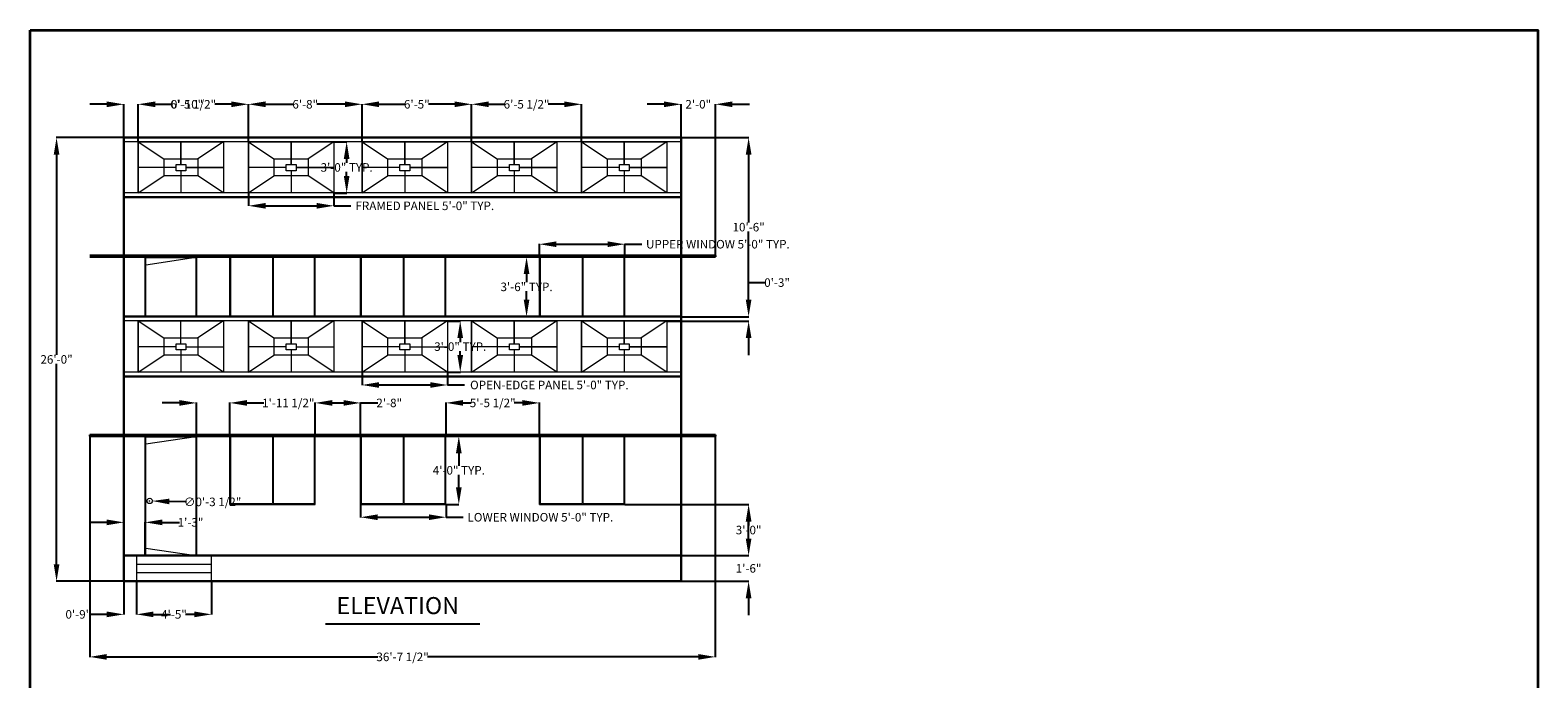
# Model space of a CAD drawing. Units: inches. Extents: x 115 to 1174, y 222 to 1302.
# Tile 5 of 5: x 115 to 1174, y 846 to 1302. Entities that reach past the tile are written whole.
import ezdxf

# ---------------------------------------------------------------- set-up
doc = ezdxf.new("R2010")
doc.units = ezdxf.units.IN
doc.header["$MEASUREMENT"] = 0
for name, color, linetype, lineweight in [('A-ANNO-DIMS', 2, 'Continuous', 18), ('A-ANNO-TEXT', 7, 'Continuous', 25), ('A-ANNO-TTLB', 7, 'Continuous', 35), ('A-ELEV', 7, 'Continuous', 30), ('A-ELEV-DOOR', 3, 'Continuous', 18), ('A-ELEV-GLAZ', 4, 'Continuous', 18), ('A-ELEV-PANL', 7, 'Continuous', 18), ('A-ELEV-STEP', 7, 'Continuous', 18)]:
    doc.layers.add(name, color=color, linetype=linetype, lineweight=lineweight)
doc.styles.get("Standard").update_dxf_attribs({"font": 'arial.ttf'})
doc.dimstyles.get("Standard").update_dxf_attribs({"dimtxt": 6, "dimasz": 12, "dimexe": 0.18, "dimexo": 0.0625, "dimgap": 0.09, "dimtad": 0, "dimtih": 1, "dimtoh": 1, "dimdec": 1, "dimzin": 0, "dimdsep": 46, "dimlunit": 3, "dimtxsty": 'Standard', "dimcen": 0.09, "dimadec": 0, "dimazin": 0, "dimtfac": 1, "dimtdec": 1, "dimtofl": 0, "dimtmove": 0, "dimatfit": 3, "dimfxl": 1, "dimtolj": 1, "dimtzin": 0, "dimarcsym": 0})

# ---------------------------------------------------------------- blocks, each defined once
blk = doc.blocks.new('FASCIA-PANEL-OPEN-EDGE')
for p, q in [((0, 36), (0, 0)), ((0, 36), (18, 24)), ((30, 20), (30, 36)), ((60, 36), (42, 24)), ((60, 36), (60, 0)), ((18, 24), (18, 12)), ((42, 24), (42, 12)), ((26.6, 17.8), (0, 17.8)), ((0, 0), (18, 12)), ((30, 15.6), (30, 0)), ((33.5, 17.8), (60, 17.8)), ((60, 0), (42, 12))]:
    blk.add_line(p, q)
for points in [[(60, 0), (0, 0), (0, 36), (60, 36)], [(18, 24), (42, 24)], [(42, 12), (18, 12)]]:
    blk.add_lwpolyline(points)
blk.add_lwpolyline([(26.6, 20), (33.5, 20), (33.5, 15.6), (26.6, 15.6)], close=True)
blk = doc.blocks.new('FASCIA-PANEL-FRAMED')
for p, q in [((0, 36), (0, 0)), ((0, 36), (18, 24)), ((30, 20), (30, 36)), ((60, 36), (42, 24)), ((60, 36), (60, 0)), ((18, 24), (18, 12)), ((42, 24), (42, 12)), ((26.6, 17.8), (0, 17.8)), ((0, 0), (18, 12)), ((30, 15.6), (30, 0)), ((33.5, 17.8), (60, 17.8)), ((60, 0), (42, 12))]:
    blk.add_line(p, q)
for points in [[(0, 36), (60, 36), (60, 0), (0, 0)], [(26.6, 20), (33.5, 20), (33.5, 15.6), (26.6, 15.6)]]:
    blk.add_lwpolyline(points, close=True)
for points in [[(18, 24), (42, 24)], [(42, 12), (18, 12)]]:
    blk.add_lwpolyline(points)
blk = doc.blocks.new('ELEV-WIN-TWIN-60X48')
for p, q in [((0, 48), (0, 0)), ((0, 0), (0, 48)), ((0.5, 47.5), (0.5, 0.5)), ((30, 47.5), (0.5, 47.5)), ((30, 47.5), (30, 0.5)), ((59.5, 47.5), (30.5, 47.5)), ((30.5, 47.5), (30.5, 0.5)), ((59.5, 0.5), (59.5, 47.5)), ((60, 0), (60, 48)), ((60, 0), (60, 48)), ((0.5, 0.5), (30, 0.5)), ((30.5, 0.5), (59.5, 0.5)), ((0, 0), (60, 0))]:
    blk.add_line(p, q)
blk = doc.blocks.new('ELEV-WIN-TWIN-60-UPPER')
for p, q in [((0, 42), (0, 0)), ((0, 0), (0, 42)), ((30, 41.5), (0.5, 41.5)), ((0.5, 41.5), (0.5, 0)), ((30, 41.5), (30, 0)), ((59.5, 41.5), (30.5, 41.5)), ((30.5, 41.5), (30.5, 0)), ((59.5, 0), (59.5, 41.5)), ((60, 0), (60, 42)), ((60, 0), (60, 42))]:
    blk.add_line(p, q)
blk = doc.blocks.new('*D29')
at = {"layer": 'A-ANNO-DIMS', "color": 0, "lineweight": -2, "transparency": 16777216}
for p, q in [((268.2, 1187.6), (268.2, 1178.5)), ((328.2, 1187.6), (328.2, 1178.5)), ((280.2, 1178.6), (316.2, 1178.6)), ((328.2, 1178.6), (340.2, 1178.6))]:
    blk.add_line(p, q, dxfattribs=at)
at = {"layer": 'A-ANNO-DIMS', "color": 0, "transparency": 16777216}
for points in [[(280.2, 1180.6), (280.2, 1176.6), (268.2, 1178.6)], [(316.2, 1180.6), (316.2, 1176.6), (328.2, 1178.6)]]:
    blk.add_solid(points, dxfattribs=at)
at = {"layer": 'Defpoints', "color": 0, "transparency": 16777216}
for p in [(268.2, 1187.6), (328.2, 1187.6), (328.2, 1178.6)]:
    blk.add_point(p, dxfattribs=at)
at = {"layer": 'A-ANNO-DIMS', "color": 0, "transparency": 16777216, "insert": (392.1, 1178.6), "char_height": 6, "attachment_point": 5}
blk.add_mtext('\\A1;FRAMED PANEL 5\'-0" TYP.', dxfattribs=at)
blk = doc.blocks.new('*D30')
at = {"layer": 'A-ANNO-DIMS', "color": 0, "lineweight": -2, "transparency": 16777216}
for p, q in [((328.2, 1223.6), (337.3, 1223.6)), ((337.2, 1211.6), (337.2, 1208.8)), ((337.2, 1199.6), (337.2, 1202.5)), ((328.2, 1187.6), (337.3, 1187.6))]:
    blk.add_line(p, q, dxfattribs=at)
at = {"layer": 'A-ANNO-DIMS', "color": 0, "transparency": 16777216}
for points in [[(335.2, 1211.6), (339.2, 1211.6), (337.2, 1223.6)], [(335.2, 1199.6), (339.2, 1199.6), (337.2, 1187.6)]]:
    blk.add_solid(points, dxfattribs=at)
at = {"layer": 'Defpoints', "color": 0, "transparency": 16777216}
for p in [(328.2, 1223.6), (337.2, 1223.6), (328.2, 1187.6)]:
    blk.add_point(p, dxfattribs=at)
at = {"layer": 'A-ANNO-DIMS', "color": 0, "transparency": 16777216, "insert": (337.2, 1205.6), "char_height": 6, "attachment_point": 5}
blk.add_mtext('\\A1;3\'-0" TYP.', dxfattribs=at)
blk = doc.blocks.new('*D31')
at = {"layer": 'A-ANNO-DIMS', "color": 0, "lineweight": -2, "transparency": 16777216}
for p, q in [((348, 1061.6), (348, 1052.5)), ((408, 1061.6), (408, 1052.5)), ((360, 1052.6), (396, 1052.6)), ((408, 1052.6), (420, 1052.6))]:
    blk.add_line(p, q, dxfattribs=at)
at = {"layer": 'A-ANNO-DIMS', "color": 0, "transparency": 16777216}
for points in [[(360, 1054.6), (360, 1050.6), (348, 1052.6)], [(396, 1054.6), (396, 1050.6), (408, 1052.6)]]:
    blk.add_solid(points, dxfattribs=at)
at = {"layer": 'Defpoints', "color": 0, "transparency": 16777216}
for p in [(348, 1061.6), (408, 1061.6), (408, 1052.6)]:
    blk.add_point(p, dxfattribs=at)
at = {"layer": 'A-ANNO-DIMS', "color": 0, "transparency": 16777216, "insert": (479.6, 1052.6), "char_height": 6, "attachment_point": 5}
blk.add_mtext('\\A1;OPEN-EDGE PANEL 5\'-0" TYP.', dxfattribs=at)
blk = doc.blocks.new('*D32')
at = {"layer": 'A-ANNO-DIMS', "color": 0, "lineweight": -2, "transparency": 16777216}
for p, q in [((408.1, 1097.6), (417.2, 1097.6)), ((417, 1085.6), (417, 1082.8)), ((417, 1073.6), (417, 1076.5)), ((408.1, 1061.6), (417.2, 1061.6))]:
    blk.add_line(p, q, dxfattribs=at)
at = {"layer": 'A-ANNO-DIMS', "color": 0, "transparency": 16777216}
for points in [[(415, 1085.6), (419, 1085.6), (417, 1097.6)], [(415, 1073.6), (419, 1073.6), (417, 1061.6)]]:
    blk.add_solid(points, dxfattribs=at)
at = {"layer": 'Defpoints', "color": 0, "transparency": 16777216}
for p in [(408, 1097.6), (417, 1097.6), (408, 1061.6)]:
    blk.add_point(p, dxfattribs=at)
at = {"layer": 'A-ANNO-DIMS', "color": 0, "transparency": 16777216, "insert": (417, 1079.6), "char_height": 6, "attachment_point": 5}
blk.add_mtext('\\A1;3\'-0" TYP.', dxfattribs=at)
blk = doc.blocks.new('*D33')
at = {"layer": 'A-ANNO-DIMS', "color": 0, "lineweight": -2, "transparency": 16777216}
for p, q in [((347, 968.6), (347, 959.5)), ((407, 968.6), (407, 959.5)), ((359, 959.6), (395, 959.6)), ((407, 959.6), (419, 959.6))]:
    blk.add_line(p, q, dxfattribs=at)
at = {"layer": 'A-ANNO-DIMS', "color": 0, "transparency": 16777216}
for points in [[(359, 961.6), (359, 957.6), (347, 959.6)], [(395, 961.6), (395, 957.6), (407, 959.6)]]:
    blk.add_solid(points, dxfattribs=at)
at = {"layer": 'Defpoints', "color": 0, "transparency": 16777216}
for p in [(347, 968.6), (407, 968.6), (407, 959.6)]:
    blk.add_point(p, dxfattribs=at)
at = {"layer": 'A-ANNO-DIMS', "color": 0, "transparency": 16777216, "insert": (473.3, 959.6), "char_height": 6, "attachment_point": 5}
blk.add_mtext('\\A1;LOWER WINDOW 5\'-0" TYP.', dxfattribs=at)
blk = doc.blocks.new('*D34')
at = {"layer": 'A-ANNO-DIMS', "color": 0, "lineweight": -2, "transparency": 16777216}
for p, q in [((407, 1016.6), (416.1, 1016.6)), ((416, 1004.6), (416, 995.8)), ((416, 980.6), (416, 989.5)), ((407, 968.6), (416.1, 968.6))]:
    blk.add_line(p, q, dxfattribs=at)
at = {"layer": 'A-ANNO-DIMS', "color": 0, "transparency": 16777216}
for points in [[(414, 1004.6), (418, 1004.6), (416, 1016.6)], [(414, 980.6), (418, 980.6), (416, 968.6)]]:
    blk.add_solid(points, dxfattribs=at)
at = {"layer": 'Defpoints', "color": 0, "transparency": 16777216}
for p in [(407, 1016.6), (416, 1016.6), (407, 968.6)]:
    blk.add_point(p, dxfattribs=at)
at = {"layer": 'A-ANNO-DIMS', "color": 0, "transparency": 16777216, "insert": (416, 992.6), "char_height": 6, "attachment_point": 5}
blk.add_mtext('\\A1;4\'-0" TYP.', dxfattribs=at)
blk = doc.blocks.new('*D35')
at = {"layer": 'A-ANNO-DIMS', "color": 0, "lineweight": -2, "transparency": 16777216}
for p, q in [((472.6, 1142.7), (472.6, 1151.8)), ((484.6, 1151.6), (520.6, 1151.6)), ((532.6, 1142.7), (532.6, 1151.8)), ((532.6, 1151.6), (544.6, 1151.6))]:
    blk.add_line(p, q, dxfattribs=at)
at = {"layer": 'A-ANNO-DIMS', "color": 0, "transparency": 16777216}
for points in [[(484.6, 1153.6), (484.6, 1149.6), (472.6, 1151.6)], [(520.6, 1153.6), (520.6, 1149.6), (532.6, 1151.6)]]:
    blk.add_solid(points, dxfattribs=at)
at = {"layer": 'Defpoints', "color": 0, "transparency": 16777216}
for p in [(532.6, 1151.6), (472.6, 1142.6), (532.6, 1142.6)]:
    blk.add_point(p, dxfattribs=at)
at = {"layer": 'A-ANNO-DIMS', "color": 0, "transparency": 16777216, "insert": (598, 1151.6), "char_height": 6, "attachment_point": 5}
blk.add_mtext('\\A1;UPPER WINDOW 5\'-0" TYP.', dxfattribs=at)
blk = doc.blocks.new('*D36')
at = {"layer": 'A-ANNO-DIMS', "color": 0, "lineweight": -2, "transparency": 16777216}
for p, q in [((472.5, 1142.6), (463.4, 1142.6)), ((463.6, 1130.6), (463.6, 1124.8)), ((463.6, 1112.6), (463.6, 1118.5)), ((472.5, 1100.6), (463.4, 1100.6))]:
    blk.add_line(p, q, dxfattribs=at)
at = {"layer": 'A-ANNO-DIMS', "color": 0, "transparency": 16777216}
for points in [[(461.6, 1130.6), (465.6, 1130.6), (463.6, 1142.6)], [(461.6, 1112.6), (465.6, 1112.6), (463.6, 1100.6)]]:
    blk.add_solid(points, dxfattribs=at)
at = {"layer": 'Defpoints', "color": 0, "transparency": 16777216}
for p in [(463.6, 1142.6), (472.6, 1142.6), (472.6, 1100.6)]:
    blk.add_point(p, dxfattribs=at)
at = {"layer": 'A-ANNO-DIMS', "color": 0, "transparency": 16777216, "insert": (463.6, 1121.6), "char_height": 6, "attachment_point": 5}
blk.add_mtext('\\A1;3\'-6" TYP.', dxfattribs=at)
blk = doc.blocks.new('*D71')
at = {"layer": 'A-ANNO-DIMS', "color": 0, "lineweight": -2, "transparency": 16777216}
for p, q in [((156.7, 1017.6), (156.7, 861.2)), ((596.2, 1017.6), (596.2, 861.2)), ((168.7, 861.4), (359.1, 861.4)), ((584.2, 861.4), (393.9, 861.4))]:
    blk.add_line(p, q, dxfattribs=at)
at = {"layer": 'A-ANNO-DIMS', "color": 0, "transparency": 16777216}
for points in [[(168.7, 863.4), (168.7, 859.4), (156.7, 861.4)], [(584.2, 863.4), (584.2, 859.4), (596.2, 861.4)]]:
    blk.add_solid(points, dxfattribs=at)
at = {"layer": 'Defpoints', "color": 0, "transparency": 16777216}
for p in [(156.7, 1017.6), (596.2, 1017.6), (596.2, 861.4)]:
    blk.add_point(p, dxfattribs=at)
at = {"layer": 'A-ANNO-DIMS', "color": 0, "transparency": 16777216, "insert": (376.5, 861.4), "char_height": 6, "attachment_point": 5}
blk.add_mtext('\\A1;36\'-7 1/2"', dxfattribs=at)
blk = doc.blocks.new('*D72')
at = {"layer": 'A-ANNO-DIMS', "color": 0, "lineweight": -2, "transparency": 16777216}
for p, q in [((180.7, 1226.6), (133.2, 1226.6)), ((133.4, 1214.6), (133.4, 1073.8)), ((133.4, 926.6), (133.4, 1067.5)), ((180.7, 914.6), (133.2, 914.6))]:
    blk.add_line(p, q, dxfattribs=at)
at = {"layer": 'A-ANNO-DIMS', "color": 0, "transparency": 16777216}
for points in [[(131.4, 1214.6), (135.4, 1214.6), (133.4, 1226.6)], [(131.4, 926.6), (135.4, 926.6), (133.4, 914.6)]]:
    blk.add_solid(points, dxfattribs=at)
at = {"layer": 'Defpoints', "color": 0, "transparency": 16777216}
for p in [(133.4, 1226.6), (180.7, 1226.6), (180.7, 914.6)]:
    blk.add_point(p, dxfattribs=at)
at = {"layer": 'A-ANNO-DIMS', "color": 0, "transparency": 16777216, "insert": (133.4, 1070.6), "char_height": 6, "attachment_point": 5}
blk.add_mtext('\\A1;26\'-0"', dxfattribs=at)
blk = doc.blocks.new('*D73')
at = {"layer": 'A-ANNO-DIMS', "color": 0, "lineweight": -2, "transparency": 16777216}
for p, q in [((560.219665, 1249.999861), (548.219665, 1249.999861)), ((572.219665, 1226.712361), (572.219665, 1250.179861)), ((596.219665, 1143.712361), (596.219665, 1250.179861)), ((608.219665, 1249.999861), (620.219665, 1249.999861))]:
    blk.add_line(p, q, dxfattribs=at)
at = {"layer": 'A-ANNO-DIMS', "color": 0, "transparency": 16777216}
for points in [[(560.219665, 1251.999861), (560.219665, 1247.999861), (572.219665, 1249.999861)], [(608.219665, 1251.999861), (608.219665, 1247.999861), (596.219665, 1249.999861)]]:
    blk.add_solid(points, dxfattribs=at)
at = {"layer": 'Defpoints', "color": 0, "transparency": 16777216}
for p in [(572.219665, 1249.999861), (572.219665, 1226.649861), (596.219665, 1143.649861)]:
    blk.add_point(p, dxfattribs=at)
at = {"layer": 'A-ANNO-DIMS', "color": 0, "transparency": 16777216, "insert": (584.219665, 1249.999861), "char_height": 6, "attachment_point": 5}
blk.add_mtext('\\A1;2\'-0"', dxfattribs=at)
blk = doc.blocks.new('*D74')
at = {"layer": 'A-ANNO-DIMS', "color": 0, "lineweight": -2, "transparency": 16777216}
for p, q in [((168.7, 1250), (156.7, 1250)), ((180.7, 1226.7), (180.7, 1250.2)), ((190.7, 1223.7), (190.7, 1250.2)), ((202.7, 1250), (214.7, 1250))]:
    blk.add_line(p, q, dxfattribs=at)
at = {"layer": 'A-ANNO-DIMS', "color": 0, "transparency": 16777216}
for points in [[(168.7, 1252), (168.7, 1248), (180.7, 1250)], [(202.7, 1252), (202.7, 1248), (190.7, 1250)]]:
    blk.add_solid(points, dxfattribs=at)
at = {"layer": 'Defpoints', "color": 0, "transparency": 16777216}
for p in [(190.7, 1250), (180.7, 1226.6), (190.7, 1223.6)]:
    blk.add_point(p, dxfattribs=at)
at = {"layer": 'A-ANNO-DIMS', "color": 0, "transparency": 16777216, "insert": (225.1, 1250), "char_height": 6, "attachment_point": 5}
blk.add_mtext('\\A1;0\'-10"', dxfattribs=at)
blk = doc.blocks.new('*D75')
at = {"layer": 'A-ANNO-DIMS', "color": 0, "lineweight": -2, "transparency": 16777216}
for p, q in [((190.7, 1223.7), (190.7, 1250.2)), ((202.7, 1250), (214.4, 1250)), ((256.2, 1250), (244.5, 1250)), ((268.2, 1223.7), (268.2, 1250.2))]:
    blk.add_line(p, q, dxfattribs=at)
at = {"layer": 'A-ANNO-DIMS', "color": 0, "transparency": 16777216}
for points in [[(202.7, 1252), (202.7, 1248), (190.7, 1250)], [(256.2, 1252), (256.2, 1248), (268.2, 1250)]]:
    blk.add_solid(points, dxfattribs=at)
at = {"layer": 'Defpoints', "color": 0, "transparency": 16777216}
for p in [(268.2, 1250), (190.7, 1223.6), (268.2, 1223.6)]:
    blk.add_point(p, dxfattribs=at)
at = {"layer": 'A-ANNO-DIMS', "color": 0, "transparency": 16777216, "insert": (229.4, 1250), "char_height": 6, "attachment_point": 5}
blk.add_mtext('\\A1;6\'-5 1/2"', dxfattribs=at)
blk = doc.blocks.new('*D76')
at = {"layer": 'A-ANNO-DIMS', "color": 0, "lineweight": -2, "transparency": 16777216}
for p, q in [((268.2, 1223.7), (268.2, 1250.2)), ((280.2, 1250), (300, 1250)), ((336, 1250), (316.2, 1250)), ((348, 1223.7), (348, 1250.2))]:
    blk.add_line(p, q, dxfattribs=at)
at = {"layer": 'A-ANNO-DIMS', "color": 0, "transparency": 16777216}
for points in [[(280.2, 1252), (280.2, 1248), (268.2, 1250)], [(336, 1252), (336, 1248), (348, 1250)]]:
    blk.add_solid(points, dxfattribs=at)
at = {"layer": 'Defpoints', "color": 0, "transparency": 16777216}
for p in [(348, 1250), (268.2, 1223.6), (348, 1223.6)]:
    blk.add_point(p, dxfattribs=at)
at = {"layer": 'A-ANNO-DIMS', "color": 0, "transparency": 16777216, "insert": (308.1, 1250), "char_height": 6, "attachment_point": 5}
blk.add_mtext('\\A1;6\'-8"', dxfattribs=at)
blk = doc.blocks.new('*D77')
at = {"layer": 'A-ANNO-DIMS', "color": 0, "lineweight": -2, "transparency": 16777216}
for p, q in [((348, 1223.7), (348, 1250.2)), ((360, 1250), (378.4, 1250)), ((413, 1250), (394.6, 1250)), ((425, 1223.7), (425, 1250.2))]:
    blk.add_line(p, q, dxfattribs=at)
at = {"layer": 'A-ANNO-DIMS', "color": 0, "transparency": 16777216}
for points in [[(360, 1252), (360, 1248), (348, 1250)], [(413, 1252), (413, 1248), (425, 1250)]]:
    blk.add_solid(points, dxfattribs=at)
at = {"layer": 'Defpoints', "color": 0, "transparency": 16777216}
for p in [(425, 1250), (348, 1223.6), (425, 1223.6)]:
    blk.add_point(p, dxfattribs=at)
at = {"layer": 'A-ANNO-DIMS', "color": 0, "transparency": 16777216, "insert": (386.5, 1250), "char_height": 6, "attachment_point": 5}
blk.add_mtext('\\A1;6\'-5"', dxfattribs=at)
blk = doc.blocks.new('*D78')
at = {"layer": 'A-ANNO-DIMS', "color": 0, "lineweight": -2, "transparency": 16777216}
for p, q in [((425, 1223.7), (425, 1250.2)), ((437, 1250), (448.5, 1250)), ((490.2, 1250), (478.7, 1250)), ((502.2, 1223.7), (502.2, 1250.2))]:
    blk.add_line(p, q, dxfattribs=at)
at = {"layer": 'A-ANNO-DIMS', "color": 0, "transparency": 16777216}
for points in [[(437, 1252), (437, 1248), (425, 1250)], [(490.2, 1252), (490.2, 1248), (502.2, 1250)]]:
    blk.add_solid(points, dxfattribs=at)
at = {"layer": 'Defpoints', "color": 0, "transparency": 16777216}
for p in [(502.2, 1250), (425, 1223.6), (502.2, 1223.6)]:
    blk.add_point(p, dxfattribs=at)
at = {"layer": 'A-ANNO-DIMS', "color": 0, "transparency": 16777216, "insert": (463.6, 1250), "char_height": 6, "attachment_point": 5}
blk.add_mtext('\\A1;6\'-5 1/2"', dxfattribs=at)
blk = doc.blocks.new('*D79')
at = {"layer": 'A-ANNO-DIMS', "color": 0, "lineweight": -2, "transparency": 16777216}
for p, q in [((180.7, 914.6), (180.7, 891.1)), ((189.5, 914.6), (189.5, 891.1)), ((168.7, 891.3), (156.7, 891.3)), ((201.5, 891.3), (213.5, 891.3))]:
    blk.add_line(p, q, dxfattribs=at)
at = {"layer": 'A-ANNO-DIMS', "color": 0, "transparency": 16777216}
for points in [[(168.7, 893.3), (168.7, 889.3), (180.7, 891.3)], [(201.5, 893.3), (201.5, 889.3), (189.5, 891.3)]]:
    blk.add_solid(points, dxfattribs=at)
at = {"layer": 'Defpoints', "color": 0, "transparency": 16777216}
for p in [(180.7, 914.6), (189.5, 914.6), (180.7, 891.3)]:
    blk.add_point(p, dxfattribs=at)
at = {"layer": 'A-ANNO-DIMS', "color": 0, "transparency": 16777216, "insert": (148.7, 891.3), "char_height": 6, "attachment_point": 5}
blk.add_mtext('\\A1;0\'-9"', dxfattribs=at)
blk = doc.blocks.new('*D80')
at = {"layer": 'A-ANNO-DIMS', "color": 0, "lineweight": -2, "transparency": 16777216}
for p, q in [((189.5, 914.6), (189.5, 891.1)), ((242.3, 914.6), (242.3, 891.1)), ((201.5, 891.3), (207.7, 891.3)), ((230.3, 891.3), (224.1, 891.3))]:
    blk.add_line(p, q, dxfattribs=at)
at = {"layer": 'A-ANNO-DIMS', "color": 0, "transparency": 16777216}
for points in [[(201.5, 893.3), (201.5, 889.3), (189.5, 891.3)], [(230.3, 893.3), (230.3, 889.3), (242.3, 891.3)]]:
    blk.add_solid(points, dxfattribs=at)
at = {"layer": 'Defpoints', "color": 0, "transparency": 16777216}
for p in [(189.5, 914.6), (242.3, 914.6), (189.5, 891.3)]:
    blk.add_point(p, dxfattribs=at)
at = {"layer": 'A-ANNO-DIMS', "color": 0, "transparency": 16777216, "insert": (215.9, 891.3), "char_height": 6, "attachment_point": 5}
blk.add_mtext('\\A1;4\'-5"', dxfattribs=at)
blk = doc.blocks.new('*D81')
at = {"layer": 'A-ANNO-DIMS', "color": 0, "lineweight": -2, "transparency": 16777216}
for p, q in [((168.7, 956), (156.7, 956)), ((180.7, 932.7), (180.7, 956.2)), ((195.7, 932.7), (195.7, 956.2)), ((207.7, 956), (219.7, 956))]:
    blk.add_line(p, q, dxfattribs=at)
at = {"layer": 'A-ANNO-DIMS', "color": 0, "transparency": 16777216}
for points in [[(168.7, 958), (168.7, 954), (180.7, 956)], [(207.7, 958), (207.7, 954), (195.7, 956)]]:
    blk.add_solid(points, dxfattribs=at)
at = {"layer": 'Defpoints', "color": 0, "transparency": 16777216}
for p in [(195.7, 956), (180.7, 932.6), (195.7, 932.6)]:
    blk.add_point(p, dxfattribs=at)
at = {"layer": 'A-ANNO-DIMS', "color": 0, "transparency": 16777216, "insert": (227.5, 956), "char_height": 6, "attachment_point": 5}
blk.add_mtext('\\A1;1\'-3"', dxfattribs=at)
blk = doc.blocks.new('*D82')
at = {"layer": 'A-ANNO-DIMS', "color": 0, "lineweight": -2, "transparency": 16777216}
for p, q in [((219.7, 1040), (207.7, 1040)), ((231.7, 1016.7), (231.7, 1040.2)), ((255.1, 1016.7), (255.1, 1040.2)), ((267.1, 1040), (279.1, 1040))]:
    blk.add_line(p, q, dxfattribs=at)
at = {"layer": 'A-ANNO-DIMS', "color": 0, "transparency": 16777216}
for points in [[(219.7, 1042), (219.7, 1038), (231.7, 1040)], [(267.1, 1042), (267.1, 1038), (255.1, 1040)]]:
    blk.add_solid(points, dxfattribs=at)
at = {"layer": 'Defpoints', "color": 0, "transparency": 16777216}
for p in [(255.1, 1040), (231.7, 1016.6), (255.1, 1016.6)]:
    blk.add_point(p, dxfattribs=at)
at = {"layer": 'A-ANNO-DIMS', "color": 0, "transparency": 16777216, "insert": (296.2, 1040), "char_height": 6, "attachment_point": 5}
blk.add_mtext('\\A1;1\'-11 1/2"', dxfattribs=at)
blk = doc.blocks.new('*D83')
at = {"layer": 'A-ANNO-DIMS', "color": 0, "lineweight": -2, "transparency": 16777216}
for p, q in [((315.1, 1016.7), (315.1, 1040.2)), ((327.1, 1040), (335, 1040)), ((347, 1016.7), (347, 1040.2)), ((347, 1040), (359, 1040))]:
    blk.add_line(p, q, dxfattribs=at)
at = {"layer": 'A-ANNO-DIMS', "color": 0, "transparency": 16777216}
for points in [[(327.1, 1042), (327.1, 1038), (315.1, 1040)], [(335, 1042), (335, 1038), (347, 1040)]]:
    blk.add_solid(points, dxfattribs=at)
at = {"layer": 'Defpoints', "color": 0, "transparency": 16777216}
for p in [(347, 1040), (315.1, 1016.6), (347, 1016.6)]:
    blk.add_point(p, dxfattribs=at)
at = {"layer": 'A-ANNO-DIMS', "color": 0, "transparency": 16777216, "insert": (367.1, 1040), "char_height": 6, "attachment_point": 5}
blk.add_mtext('\\A1;2\'-8"', dxfattribs=at)
blk = doc.blocks.new('*D84')
at = {"layer": 'A-ANNO-DIMS', "color": 0, "lineweight": -2, "transparency": 16777216}
for p, q in [((407, 1016.7), (407, 1040.2)), ((419, 1040), (424.7, 1040)), ((460.6, 1040), (454.8, 1040)), ((472.6, 1016.7), (472.6, 1040.2))]:
    blk.add_line(p, q, dxfattribs=at)
at = {"layer": 'A-ANNO-DIMS', "color": 0, "transparency": 16777216}
for points in [[(419, 1042), (419, 1038), (407, 1040)], [(460.6, 1042), (460.6, 1038), (472.6, 1040)]]:
    blk.add_solid(points, dxfattribs=at)
at = {"layer": 'Defpoints', "color": 0, "transparency": 16777216}
for p in [(472.6, 1040), (407, 1016.6), (472.6, 1016.6)]:
    blk.add_point(p, dxfattribs=at)
at = {"layer": 'A-ANNO-DIMS', "color": 0, "transparency": 16777216, "insert": (439.8, 1040), "char_height": 6, "attachment_point": 5}
blk.add_mtext('\\A1;5\'-5 1/2"', dxfattribs=at)
blk = doc.blocks.new('*D85')
at = {"layer": 'A-ANNO-DIMS', "color": 0, "lineweight": -2, "transparency": 16777216}
for p, q in [((619.569665, 944.649861), (619.569665, 956.649861)), ((572.282165, 932.649861), (619.749665, 932.649861)), ((572.282165, 914.649861), (619.749665, 914.649861)), ((619.569665, 902.649861), (619.569665, 890.649861))]:
    blk.add_line(p, q, dxfattribs=at)
at = {"layer": 'A-ANNO-DIMS', "color": 0, "transparency": 16777216}
for points in [[(617.569665, 944.649861), (621.569665, 944.649861), (619.569665, 932.649861)], [(617.569665, 902.649861), (621.569665, 902.649861), (619.569665, 914.649861)]]:
    blk.add_solid(points, dxfattribs=at)
at = {"layer": 'Defpoints', "color": 0, "transparency": 16777216}
for p in [(572.219665, 932.649861), (619.569665, 932.649861), (572.219665, 914.649861)]:
    blk.add_point(p, dxfattribs=at)
at = {"layer": 'A-ANNO-DIMS', "color": 0, "transparency": 16777216, "insert": (619.569665, 923.649861), "char_height": 6, "attachment_point": 5}
blk.add_mtext('\\A1;1\'-6"', dxfattribs=at)
blk = doc.blocks.new('*D86')
at = {"layer": 'A-ANNO-DIMS', "color": 0, "lineweight": -2, "transparency": 16777216}
for p, q in [((532.7, 968.6), (619.7, 968.6)), ((619.6, 956.6), (619.6, 953.8)), ((619.6, 944.6), (619.6, 947.5)), ((572.3, 932.6), (619.7, 932.6))]:
    blk.add_line(p, q, dxfattribs=at)
at = {"layer": 'A-ANNO-DIMS', "color": 0, "transparency": 16777216}
for points in [[(617.6, 956.6), (621.6, 956.6), (619.6, 968.6)], [(617.6, 944.6), (621.6, 944.6), (619.6, 932.6)]]:
    blk.add_solid(points, dxfattribs=at)
at = {"layer": 'Defpoints', "color": 0, "transparency": 16777216}
for p in [(532.6, 968.6), (619.6, 968.6), (572.2, 932.6)]:
    blk.add_point(p, dxfattribs=at)
at = {"layer": 'A-ANNO-DIMS', "color": 0, "transparency": 16777216, "insert": (619.6, 950.6), "char_height": 6, "attachment_point": 5}
blk.add_mtext('\\A1;3\'-0"', dxfattribs=at)
blk = doc.blocks.new('*D87')
at = {"layer": 'A-ANNO-DIMS', "color": 0, "lineweight": -2, "transparency": 16777216}
for p, q in [((572.3, 1226.6), (619.7, 1226.6)), ((619.6, 1214.6), (619.6, 1166.8)), ((619.6, 1112.6), (619.6, 1160.5)), ((572.3, 1100.6), (619.7, 1100.6))]:
    blk.add_line(p, q, dxfattribs=at)
at = {"layer": 'A-ANNO-DIMS', "color": 0, "transparency": 16777216}
for points in [[(617.6, 1214.6), (621.6, 1214.6), (619.6, 1226.6)], [(617.6, 1112.6), (621.6, 1112.6), (619.6, 1100.6)]]:
    blk.add_solid(points, dxfattribs=at)
at = {"layer": 'Defpoints', "color": 0, "transparency": 16777216}
for p in [(572.2, 1226.6), (619.6, 1226.6), (572.2, 1100.6)]:
    blk.add_point(p, dxfattribs=at)
at = {"layer": 'A-ANNO-DIMS', "color": 0, "transparency": 16777216, "insert": (619.6, 1163.6), "char_height": 6, "attachment_point": 5}
blk.add_mtext('\\A1;10\'-6"', dxfattribs=at)
blk = doc.blocks.new('*D88')
at = {"layer": 'A-ANNO-DIMS', "color": 0, "lineweight": -2, "transparency": 16777216}
for p, q in [((619.6, 1112.6), (619.6, 1124.6)), ((619.6, 1124.6), (631.6, 1124.6)), ((562.3, 1097.6), (619.7, 1097.6)), ((572.3, 1100.6), (619.7, 1100.6)), ((619.6, 1085.6), (619.6, 1073.6))]:
    blk.add_line(p, q, dxfattribs=at)
at = {"layer": 'A-ANNO-DIMS', "color": 0, "transparency": 16777216}
for points in [[(617.6, 1112.6), (621.6, 1112.6), (619.6, 1100.6)], [(617.6, 1085.6), (621.6, 1085.6), (619.6, 1097.6)]]:
    blk.add_solid(points, dxfattribs=at)
at = {"layer": 'Defpoints', "color": 0, "transparency": 16777216}
for p in [(562.2, 1097.6), (572.2, 1100.6), (619.6, 1100.6)]:
    blk.add_point(p, dxfattribs=at)
at = {"layer": 'A-ANNO-DIMS', "color": 0, "transparency": 16777216, "insert": (639.6, 1124.6), "char_height": 6, "attachment_point": 5}
blk.add_mtext('\\A1;0\'-3"', dxfattribs=at)
blk = doc.blocks.new('*D98')
at = {"layer": 'A-ANNO-DIMS', "color": 0, "lineweight": -2, "transparency": 16777216}
for p, q in [((198.7, 971.1), (198.9, 971.1)), ((198.8, 971), (198.8, 971.1)), ((224.7, 970.4), (212.7, 970.7))]:
    blk.add_line(p, q, dxfattribs=at)
at = {"layer": 'A-ANNO-DIMS', "color": 0, "transparency": 16777216}
blk.add_solid([(212.7, 972.7), (212.6, 968.7), (200.7, 971)], dxfattribs=at)
at = {"layer": 'Defpoints', "color": 0, "transparency": 16777216}
for p in [(197, 971.1), (200.7, 971)]:
    blk.add_point(p, dxfattribs=at)
at = {"layer": 'A-ANNO-DIMS', "color": 0, "transparency": 16777216, "insert": (243, 970.4), "char_height": 6, "attachment_point": 5}
blk.add_mtext('\\A1;∅0\'-3 1/2"', dxfattribs=at)

msp = doc.modelspace()

# ---------------------------------------------------------------- linework, layer by layer
at = {"layer": 'A-ANNO-TEXT'}
msp.add_line((322.46, 884.76), (430.72, 884.76), dxfattribs=at)
at = {"layer": 'A-ANNO-TTLB'}
msp.add_lwpolyline([(114.85, 1302.15), (1174.06, 1302.15), (1174.06, 222.13), (114.85, 222.13)], close=True, dxfattribs=at)
at = {"layer": 'A-ELEV'}
for p, q in [((572.22, 1226.65), (180.72, 1226.65)), ((180.72, 1097.65), (180.72, 1226.65)), ((572.22, 1040.65), (572.22, 1226.65)), ((572.22, 1184.65), (180.72, 1184.65)), ((156.72, 1143.65), (572.22, 1143.65)), ((180.72, 1142.65), (156.72, 1142.65)), ((572.22, 1142.65), (180.72, 1142.65)), ((572.22, 1143.65), (596.22, 1143.65)), ((596.22, 1142.65), (572.22, 1142.65)), ((596.22, 1143.65), (596.22, 1142.65)), ((180.72, 914.65), (180.72, 1100.65)), ((572.22, 1100.65), (180.72, 1100.65)), ((572.22, 914.65), (572.22, 1100.65)), ((572.22, 1058.65), (180.72, 1058.65)), ((156.72, 1016.65), (156.72, 1017.65)), ((156.72, 1017.65), (572.22, 1017.65)), ((572.22, 1017.65), (596.22, 1017.65)), ((596.22, 1017.65), (596.22, 1016.65)), ((180.72, 1016.65), (156.72, 1016.65)), ((572.22, 1016.65), (180.72, 1016.65)), ((596.22, 1016.65), (572.22, 1016.65)), ((572.22, 932.65), (180.72, 932.65)), ((572.22, 914.65), (180.72, 914.65))]:
    msp.add_line(p, q, dxfattribs=at)
at = {"layer": 'A-ELEV-DOOR'}
for p, q in [((195.72, 1142.65), (231.72, 1142.65)), ((195.72, 1100.65), (195.72, 1142.65)), ((195.72, 1100.65), (195.72, 1142.65)), ((196.22, 1142.15), (231.22, 1142.15)), ((196.22, 1100.65), (196.22, 1142.15)), ((231.22, 1142.15), (196.22, 1136.89)), ((231.22, 1142.15), (231.22, 1100.65)), ((231.72, 1142.65), (231.72, 1100.65)), ((231.72, 1100.65), (231.72, 1142.65)), ((195.72, 932.65), (195.72, 1016.65)), ((195.72, 932.65), (195.72, 1016.65)), ((195.72, 1016.65), (231.72, 1016.65)), ((196.22, 932.65), (196.22, 1016.15)), ((196.22, 1016.15), (231.22, 1016.15)), ((231.22, 1016.15), (196.22, 1010.89)), ((231.22, 1016.15), (231.22, 932.65)), ((231.72, 932.65), (231.72, 1016.65)), ((231.72, 1016.65), (231.72, 932.65)), ((196.22, 932.65), (196.22, 937.95)), ((196.22, 937.95), (231.22, 932.65))]:
    msp.add_line(p, q, dxfattribs=at)
msp.add_circle((198.83, 971.05), 1.87, dxfattribs=at)
at = {"layer": 'A-ELEV-GLAZ'}
for p, q in [((406.96, 1142.65), (346.96, 1142.65)), ((532.61, 1142.65), (472.61, 1142.65)), ((406.96, 1016.65), (346.96, 1016.65)), ((532.61, 1016.65), (472.61, 1016.65))]:
    msp.add_line(p, q, dxfattribs=at)
at = {"layer": 'A-ELEV-PANL'}
for p, q in [((572.22, 1223.65), (180.72, 1223.65)), ((180.72, 1223.65), (180.72, 1187.65)), ((220.72, 1223.65), (220.72, 1207.7)), ((298.15, 1223.65), (298.15, 1207.7)), ((378.01, 1223.65), (378.01, 1207.7)), ((454.96, 1223.65), (454.96, 1207.7)), ((532.22, 1223.65), (532.22, 1207.7)), ((562.22, 1223.65), (562.22, 1187.65)), ((572.22, 1223.65), (572.22, 1187.65)), ((250.72, 1205.45), (224.25, 1205.45)), ((328.15, 1205.45), (301.69, 1205.45)), ((408.01, 1205.45), (381.55, 1205.45)), ((484.96, 1205.45), (458.49, 1205.45)), ((562.22, 1205.45), (535.75, 1205.45)), ((572.22, 1187.65), (180.72, 1187.65)), ((572.22, 1097.65), (180.72, 1097.65)), ((180.72, 1097.65), (180.72, 1061.65)), ((298.15, 1097.65), (298.15, 1081.7)), ((378.01, 1097.65), (378.01, 1081.7)), ((454.96, 1097.65), (454.96, 1081.7)), ((532.22, 1097.65), (532.22, 1081.7)), ((562.22, 1097.65), (562.22, 1061.65)), ((572.22, 1097.65), (572.22, 1061.65)), ((484.96, 1079.45), (458.49, 1079.45)), ((562.22, 1079.45), (535.75, 1079.45)), ((572.22, 1061.65), (180.72, 1061.65)), ((180.72, 1058.65), (180.72, 1061.65))]:
    msp.add_line(p, q, dxfattribs=at)
at = {"layer": 'A-ELEV-STEP'}
for p, q in [((189.5, 932.65), (189.5, 914.65)), ((242.31, 932.65), (189.5, 932.65)), ((242.31, 914.65), (242.31, 932.65)), ((189.5, 926.65), (242.31, 926.65)), ((189.5, 920.65), (242.31, 920.65)), ((189.5, 914.65), (242.31, 914.65))]:
    msp.add_line(p, q, dxfattribs=at)

# ---------------------------------------------------------------- block references
at = {"layer": 'A-ELEV-GLAZ'}
for name, p in [('ELEV-WIN-TWIN-60-UPPER', (255.09, 1100.65)), ('ELEV-WIN-TWIN-60-UPPER', (346.96, 1100.65)), ('ELEV-WIN-TWIN-60-UPPER', (472.61, 1100.65)), ('ELEV-WIN-TWIN-60X48', (255.09, 968.65)), ('ELEV-WIN-TWIN-60X48', (346.96, 968.65)), ('ELEV-WIN-TWIN-60X48', (472.61, 968.65))]:
    msp.add_blockref(name, p, dxfattribs=at)
at = {"layer": 'A-ELEV-PANL'}
for name, p in [('FASCIA-PANEL-FRAMED', (190.72, 1187.65)), ('FASCIA-PANEL-FRAMED', (268.16, 1187.65)), ('FASCIA-PANEL-FRAMED', (348.01, 1187.65)), ('FASCIA-PANEL-FRAMED', (424.96, 1187.65)), ('FASCIA-PANEL-FRAMED', (502.22, 1187.65)), ('FASCIA-PANEL-OPEN-EDGE', (190.72, 1061.65)), ('FASCIA-PANEL-OPEN-EDGE', (268.16, 1061.65)), ('FASCIA-PANEL-OPEN-EDGE', (348.01, 1061.65)), ('FASCIA-PANEL-FRAMED', (424.96, 1061.65)), ('FASCIA-PANEL-FRAMED', (502.22, 1061.65))]:
    msp.add_blockref(name, p, dxfattribs=at)

# ---------------------------------------------------------------- texts
at = {"layer": 'A-ANNO-TEXT', "insert": (330.02, 903.46), "char_height": 12, "attachment_point": 1}
msp.add_mtext_dynamic_manual_height_columns('ELEVATION', width=186.2726, gutter_width=30, heights=[0], dxfattribs=at)

# ---------------------------------------------------------------- dimensions: what is measured, and where the dimension line sits
at = {"layer": 'A-ANNO-DIMS'}
for base, p1, p2, picture, middle in [((190.72, 1250), (180.72, 1226.65), (190.72, 1223.65), '*D74', (225.12, 1250)), ((268.15, 1250), (190.72, 1223.65), (268.15, 1223.65), '*D75', (229.44, 1250)), ((348.01, 1250), (268.15, 1223.65), (348.01, 1223.65), '*D76', (308.08, 1250)), ((424.9597, 1249.9999), (348.0128, 1223.6499), (424.9597, 1223.6499), '*D77', (386.4862, 1249.9999)), ((502.22, 1250), (424.96, 1223.65), (502.22, 1223.65), '*D78', (463.59, 1250)), ((572.22, 1250), (596.22, 1143.65), (572.22, 1226.65), '*D73', (584.22, 1250)), ((346.96, 1040), (315.09, 1016.65), (346.96, 1016.65), '*D83', (367.07, 1040)), ((596.22, 861.41), (156.72, 1017.65), (596.22, 1017.65), '*D71', (376.47, 861.41))]:
    dim = msp.add_linear_dim(base=base, p1=p1, p2=p2, dimstyle='Standard', override={"dimdec": 1, "dimlfac": 1, "dimrnd": 0, "dimzin": 1, "dimdsep": 46, "dimlunit": 4, "dimfrac": 2}, dxfattribs=at)
    dim.commit()
    dim.dimension.update_dxf_attribs({"geometry": picture, "text_midpoint": middle})
for base, p1, p2, angle, picture, middle in [((133.37, 1226.65), (180.72, 914.65), (180.72, 1226.65), 90, '*D72', (133.37, 1070.65)), ((619.57, 1226.65), (572.22, 1100.65), (572.22, 1226.65), 90, '*D87', (619.57, 1163.65)), ((619.57, 1100.65), (562.22, 1097.65), (572.22, 1100.65), 90, '*D88', (639.63, 1124.65)), ((255.09, 1040), (231.72, 1016.65), (255.09, 1016.65), 0, '*D82', (296.19, 1040)), ((472.6086, 1039.9999), (406.9573, 1016.6499), (472.6086, 1016.6499), 0, '*D84', (439.783, 1039.9999)), ((619.57, 968.65), (572.22, 932.65), (532.61, 968.65), 90, '*D86', (619.57, 950.65)), ((195.72, 956), (180.72, 932.65), (195.72, 932.65), 0, '*D81', (227.5, 956)), ((619.57, 932.65), (572.22, 914.65), (572.22, 932.65), 90, '*D85', (619.57, 923.65)), ((180.72, 891.3), (189.5, 914.65), (180.72, 914.65), 180, '*D79', (148.65, 891.3)), ((189.5, 891.3), (242.31, 914.65), (189.5, 914.65), 180, '*D80', (215.91, 891.3))]:
    dim = msp.add_linear_dim(base=base, p1=p1, p2=p2, angle=angle, dimstyle='Standard', override={"dimdec": 1, "dimlfac": 1, "dimrnd": 0, "dimzin": 1, "dimdsep": 46, "dimlunit": 4, "dimfrac": 2}, dxfattribs=at)
    dim.commit()
    dim.dimension.update_dxf_attribs({"geometry": picture, "text_midpoint": middle})
for base, p1, p2, picture, middle in [((337.15, 1223.65), (328.15, 1187.65), (328.15, 1223.65), '*D30', (337.15, 1205.65)), ((463.61, 1142.65), (472.61, 1100.65), (472.61, 1142.65), '*D36', (463.61, 1121.65)), ((417.01, 1097.65), (408.01, 1061.65), (408.01, 1097.65), '*D32', (417.01, 1079.65)), ((415.96, 1016.65), (406.96, 968.65), (406.96, 1016.65), '*D34', (415.96, 992.65))]:
    dim = msp.add_linear_dim(base=base, p1=p1, p2=p2, angle=90, text='<> TYP.', dimstyle='Standard', override={"dimdec": 1, "dimlfac": 1, "dimrnd": 0, "dimzin": 1, "dimdsep": 46, "dimlunit": 4, "dimfrac": 2}, dxfattribs=at)
    dim.commit()
    dim.dimension.update_dxf_attribs({"geometry": picture, "text_midpoint": middle})
for base, p1, p2, text, picture, middle in [((328.15, 1178.65), (268.15, 1187.65), (328.15, 1187.65), 'FRAMED PANEL <> TYP.', '*D29', (392.13, 1178.65)), ((532.61, 1151.65), (472.61, 1142.65), (532.61, 1142.65), 'UPPER WINDOW <> TYP.', '*D35', (597.99, 1151.65)), ((408.01, 1052.65), (348.01, 1061.65), (408.01, 1061.65), 'OPEN-EDGE PANEL <> TYP.', '*D31', (479.58, 1052.65)), ((406.96, 959.65), (346.96, 968.65), (406.96, 968.65), 'LOWER WINDOW <> TYP.', '*D33', (473.29, 959.65))]:
    dim = msp.add_linear_dim(base=base, p1=p1, p2=p2, text=text, dimstyle='Standard', override={"dimdec": 1, "dimlfac": 1, "dimrnd": 0, "dimzin": 1, "dimdsep": 46, "dimlunit": 4, "dimfrac": 2}, dxfattribs=at)
    dim.commit()
    dim.dimension.update_dxf_attribs({"geometry": picture, "text_midpoint": middle})
dim = msp.add_diameter_dim_2p(p1=(196.9543, 971.1012), p2=(200.7013, 971.0026), dimstyle='Standard', override={"dimdec": 1, "dimlfac": 1, "dimrnd": 0, "dimzin": 1, "dimdsep": 46, "dimlunit": 4, "dimfrac": 2}, dxfattribs=at)
dim.commit()
dim.dimension.update_dxf_attribs({"geometry": '*D98', "text_midpoint": (224.693, 970.3712), "dimtype": 163})

doc.saveas('drawing.dxf')
